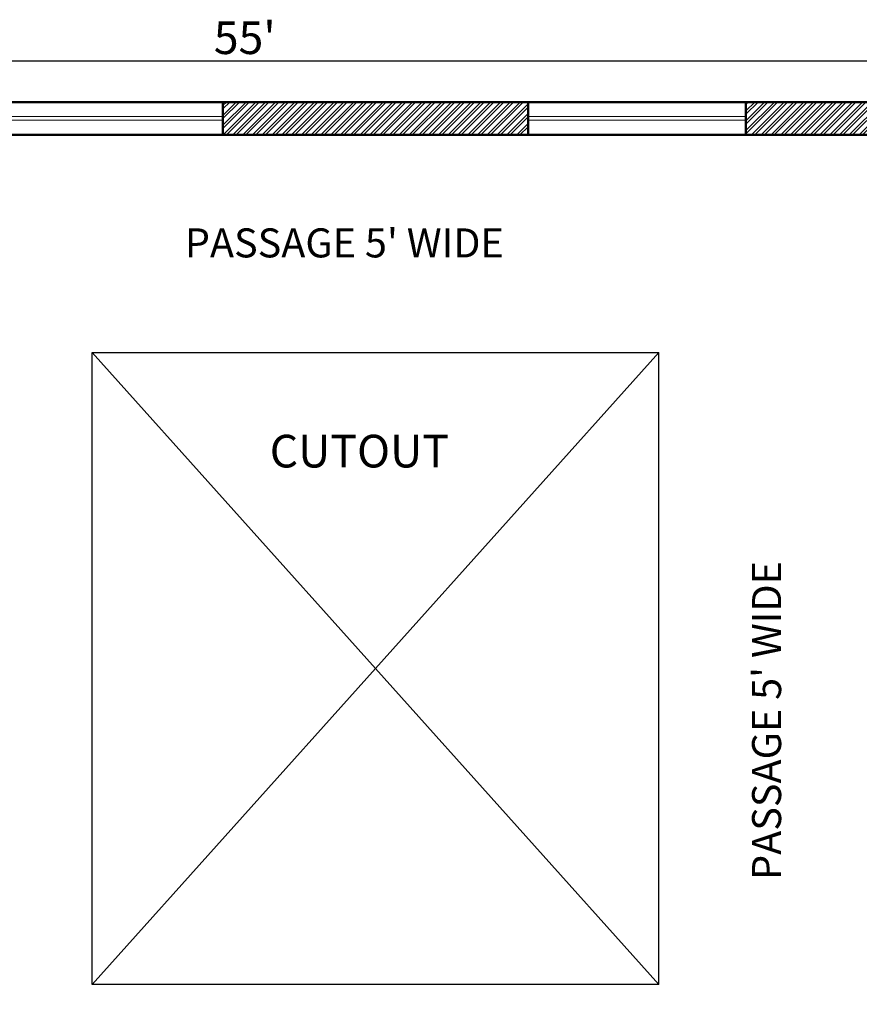
# Model space of a CAD drawing. Units: inches. Extents: x 3590 to 5167, y 65 to 1917.
# Tile 57 of 100: x 4688 to 4919, y 1558 to 1829. Entities that reach past the tile are written whole.
import ezdxf

# ---------------------------------------------------------------- set-up
doc = ezdxf.new("R2010")
doc.units = ezdxf.units.IN
for name, color, linetype, lineweight in [('A-ANNO-DIMS', 2, 'Continuous', 18), ('A-AREA-IDEN', 7, 'Continuous', 18), ('A-FLOR-OTLN', 7, 'Continuous', 25), ('A-GLAZ', 4, 'Continuous', 18), ('A-WALL', 7, 'Continuous', 50), ('A-WALL-PATT', 251, 'Continuous', 13)]:
    doc.layers.add(name, color=color, linetype=linetype, lineweight=lineweight)
doc.styles.get("Standard").update_dxf_attribs({"font": 'arial.ttf'})
doc.dimstyles.new('ISO-25', dxfattribs={"dimtxt": 9, "dimasz": 2.5, "dimexe": 1.25, "dimexo": 0.625, "dimtad": 1, "dimdec": 1, "dimlunit": 3, "dimtxsty": 'Standard', "dimcen": 2.5, "dimadec": 0, "dimazin": 0, "dimtfac": 1, "dimtdec": 1, "dimtmove": 0, "dimatfit": 3, "dimfxl": 1, "dimarcsym": 0})

# ---------------------------------------------------------------- blocks, each defined once
blk = doc.blocks.new('*D101')
at = {"layer": 'A-ANNO-DIMS', "color": 0, "lineweight": -2, "transparency": 16777216}
for p, q in [((4420.27, 1806.62), (4420.27, 1818.61)), ((4422.77, 1817.36), (5077.77, 1817.36)), ((5080.27, 1806.62), (5080.27, 1818.61))]:
    blk.add_line(p, q, dxfattribs=at)
at = {"layer": 'A-ANNO-DIMS', "color": 0, "transparency": 16777216}
for points in [[(4422.77, 1817.78), (4422.77, 1816.95), (4420.27, 1817.36)], [(5077.77, 1817.78), (5077.77, 1816.95), (5080.27, 1817.36)]]:
    blk.add_solid(points, dxfattribs=at)
at = {"layer": 'Defpoints', "color": 0, "transparency": 16777216}
for p in [(5080.27, 1817.36), (4420.27, 1806), (5080.27, 1806)]:
    blk.add_point(p, dxfattribs=at)
at = {"layer": 'A-ANNO-DIMS', "color": 0, "transparency": 16777216, "insert": (4750.27, 1822.57), "char_height": 9, "attachment_point": 5}
blk.add_mtext("55'", dxfattribs=at)

msp = doc.modelspace()

# ---------------------------------------------------------------- hatches: boundary and pattern name
at = {"layer": 'A-WALL-PATT', "transparency": 33554687}
h = msp.add_hatch(dxfattribs=at)
h.set_pattern_fill('ANSI32', color=256, scale=0.2)
h.paths.add_polyline_path([(4684.27, 1806), (4591.27, 1806), (4591.27, 1797), (4639.27, 1797), (4639.27, 1791), (4648.27, 1791), (4648.27, 1797), (4684.27, 1797)])
h.paths.add_polyline_path([(4543.27, 1806), (4420.27, 1806), (4420.27, 1785), (4429.27, 1785), (4429.27, 1797), (4445.92, 1797), (4543.27, 1797)])
h.paths.add_polyline_path([(4828.27, 1806), (4744.27, 1806), (4744.27, 1797), (4828.27, 1797)])
h.paths.add_polyline_path([(4648.27, 1755), (4639.27, 1755), (4639.27, 1656), (4546.27, 1656), (4546.27, 1650), (4549.27, 1650), (4549.27, 1554), (4429.27, 1554), (4429.27, 1584), (4420.27, 1584), (4420.27, 1539), (4429.27, 1539), (4429.27, 1545), (4639.27, 1545), (4639.27, 1539), (4648.27, 1539), (4648.27, 1560), (4639.27, 1560), (4639.27, 1554), (4555.27, 1554), (4555.27, 1650), (4639.27, 1650), (4639.27, 1590), (4648.27, 1590)])
h.paths.add_polyline_path([(4516.27, 1656), (4429.27, 1656), (4429.27, 1737), (4420.27, 1737), (4420.27, 1620), (4429.27, 1620), (4429.27, 1650), (4516.27, 1650)], flags=17)
h.paths.add_polyline_path([(5080.27, 1806), (4888.27, 1806), (4888.27, 1797), (4924.27, 1797), (4924.27, 1755), (4933.27, 1755), (4933.27, 1797), (5071.27, 1797), (5071.27, 1335), (4933.27, 1335), (4933.27, 1566), (4924.27, 1566), (4924.27, 1335), (4898.77, 1335), (4898.77, 1326), (5080.27, 1326)])
h.paths.add_polyline_path([(4933.27, 1719), (4924.27, 1719), (4924.27, 1638), (4933.27, 1638)], flags=17)
h.paths.add_polyline_path([(4802.77, 1335), (4777.27, 1335), (4777.27, 1503), (4756.27, 1503), (4756.27, 1494), (4768.27, 1494), (4768.27, 1431), (4696.27, 1431), (4696.27, 1494), (4708.27, 1494), (4708.27, 1503), (4639.27, 1503), (4639.27, 1494), (4687.27, 1494), (4687.27, 1431), (4681.27, 1431), (4681.27, 1422), (4768.27, 1422), (4768.27, 1335), (4726.27, 1335), (4726.27, 1326), (4802.77, 1326)])
h.paths.add_polyline_path([(4690.27, 1335), (4648.27, 1335), (4648.27, 1352.87), (4648.27, 1422), (4651.27, 1422), (4651.27, 1431), (4639.27, 1431), (4639.27, 1335), (4633.27, 1335), (4633.27, 1326), (4690.27, 1326)])
h.paths.add_polyline_path([(4585.27, 1335), (4584.72, 1335), (4429.27, 1335), (4429.27, 1491), (4420.27, 1491), (4420.27, 1326), (4585.27, 1326)])

# ---------------------------------------------------------------- linework, layer by layer
at = {"layer": 'A-FLOR-OTLN'}
for p, q in [((4708.27, 1563), (4708.27, 1737)), ((4708.27, 1737), (4864.27, 1737)), ((4864.27, 1563), (4864.27, 1737)), ((4864.27, 1563), (4708.27, 1563))]:
    msp.add_line(p, q, dxfattribs=at)
at = {"layer": 'A-FLOR-OTLN', "ltscale": 0.5}
for p, q in [((4708.27, 1737), (4864.27, 1563)), ((4708.27, 1563), (4864.27, 1737))]:
    msp.add_line(p, q, dxfattribs=at)
at = {"layer": 'A-GLAZ'}
for p, q in [((4744.27, 1802), (4684.27, 1802)), ((4744.27, 1801), (4684.27, 1801)), ((4888.27, 1802), (4828.27, 1802)), ((4888.27, 1801), (4828.27, 1801))]:
    msp.add_line(p, q, dxfattribs=at)
at = {"layer": 'A-WALL'}
for p, q in [((4744.27, 1797), (4744.27, 1806)), ((4828.27, 1797), (4828.27, 1806)), ((4888.27, 1797), (4888.27, 1806)), ((4648.27, 1797), (4924.27, 1797))]:
    msp.add_line(p, q, dxfattribs=at)
msp.add_lwpolyline([(5080.27, 1806), (5080.27, 1326), (4420.27, 1326), (4420.27, 1806)], close=True, dxfattribs=at)

# ---------------------------------------------------------------- texts
at = {"layer": 'A-AREA-IDEN', "attachment_point": 1}
for s, width, insert, char_height in [("{\\fTimes New Roman|b0|i0|c0|p18;PASSAGE 5' WIDE}", 131.4857, (4733.77, 1771.22), 8), ('{\\fTimes New Roman|b0|i0|c0|p18;CUTOUT}', 98.8219, (4757.14, 1714.37), 9)]:
    msp.add_mtext_dynamic_manual_height_columns(s, width=width, gutter_width=12.5, heights=[0], dxfattribs=dict(at, insert=insert, char_height=char_height))
at = {"layer": 'A-AREA-IDEN', "insert": (4889.96, 1591.77), "char_height": 8, "attachment_point": 1, "rotation": 90}
msp.add_mtext_dynamic_manual_height_columns("{\\fTimes New Roman|b0|i0|c0|p18;PASSAGE 5' WIDE}", width=131.4857, gutter_width=12.5, heights=[0], dxfattribs=at)

# ---------------------------------------------------------------- dimensions: what is measured, and where the dimension line sits
at = {"layer": 'A-ANNO-DIMS'}
dim = msp.add_linear_dim(base=(5080.27, 1817.36), p1=(4420.27, 1806), p2=(5080.27, 1806), dimstyle='ISO-25', override={"dimclrd": 0, "dimclre": 0, "dimclrt": 0}, dxfattribs=at)
dim.commit()
dim.dimension.update_dxf_attribs({"geometry": '*D101', "text_midpoint": (4750.27, 1822.57)})

doc.saveas('drawing.dxf')
